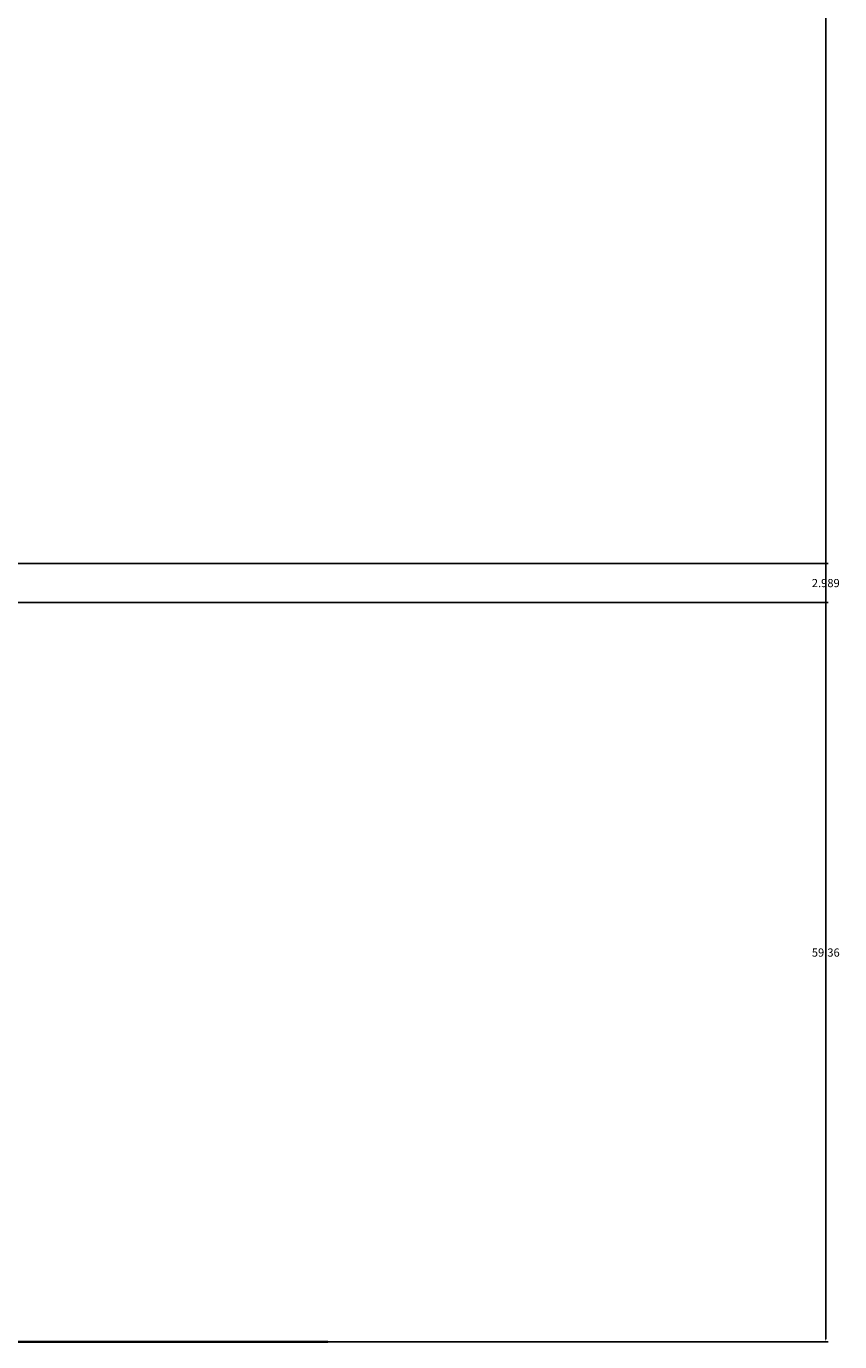
# Model space of a CAD drawing. Units: inches. Extents: x -13 to 809, y 112 to 656.
# Tile 45 of 55: x 747 to 809, y 151 to 251. Entities that reach past the tile are written whole.
import ezdxf

# ---------------------------------------------------------------- set-up
doc = ezdxf.new("R2010")
doc.units = ezdxf.units.IN
doc.header["$MEASUREMENT"] = 0
doc.layers.add('A-ANNO-DIMS', color=2, linetype='Continuous', lineweight=18)
doc.layers.add('A-ELEV', color=7, linetype='Continuous', lineweight=35)
doc.styles.get("Standard").update_dxf_attribs({"font": 'arial.ttf'})
doc.dimstyles.get("Standard").update_dxf_attribs({"dimtxt": 0.625, "dimasz": 0.18, "dimexe": 0.18, "dimexo": 0.0625, "dimgap": 0.09, "dimtad": 0, "dimtih": 1, "dimtoh": 1, "dimdec": 4, "dimzin": 0, "dimdsep": 46, "dimlunit": 4, "dimtxsty": 'Standard', "dimcen": 0.09, "dimadec": 0, "dimazin": 0, "dimtfac": 1, "dimtdec": 4, "dimtofl": 0, "dimtmove": 0, "dimatfit": 3, "dimfxl": 1, "dimtolj": 1, "dimtzin": 0, "dimarcsym": 0})

# ---------------------------------------------------------------- blocks, each defined once
blk = doc.blocks.new('*D31')
at = {"layer": 'A-ANNO-DIMS', "color": 0, "lineweight": -2, "transparency": 16777216}
for p, q in [((621.07, 617.78), (807.77, 617.78)), ((807.59, 617.6), (807.59, 384.56)), ((807.59, 150.7), (807.59, 383.74)), ((621.07, 150.52), (807.77, 150.52))]:
    blk.add_line(p, q, dxfattribs=at)
at = {"layer": 'A-ANNO-DIMS', "color": 0, "transparency": 16777216}
for points in [[(807.56, 617.6), (807.62, 617.6), (807.59, 617.78)], [(807.56, 150.7), (807.62, 150.7), (807.59, 150.52)]]:
    blk.add_solid(points, dxfattribs=at)
at = {"layer": 'Defpoints', "color": 0, "transparency": 16777216}
for p in [(621.01, 617.78), (807.59, 617.78), (621.01, 150.52)]:
    blk.add_point(p, dxfattribs=at)
at = {"layer": 'A-ANNO-DIMS', "color": 0, "transparency": 16777216, "insert": (807.59, 384.15), "char_height": 0.625, "attachment_point": 5}
blk.add_mtext('\\A1;467.3', dxfattribs=at)
blk = doc.blocks.new('*D129')
at = {"layer": 'A-ANNO-DIMS', "color": 0, "lineweight": -2, "transparency": 16777216}
for p, q in [((607.64, 209.88), (807.77, 209.88)), ((807.59, 209.7), (807.59, 180.61)), ((807.59, 150.7), (807.59, 179.79)), ((608.76, 150.52), (807.77, 150.52))]:
    blk.add_line(p, q, dxfattribs=at)
at = {"layer": 'A-ANNO-DIMS', "color": 0, "transparency": 16777216}
for points in [[(807.56, 209.7), (807.62, 209.7), (807.59, 209.88)], [(807.56, 150.7), (807.62, 150.7), (807.59, 150.52)]]:
    blk.add_solid(points, dxfattribs=at)
at = {"layer": 'Defpoints', "color": 0, "transparency": 16777216}
for p in [(607.57, 209.88), (807.59, 209.88), (608.69, 150.52)]:
    blk.add_point(p, dxfattribs=at)
at = {"layer": 'A-ANNO-DIMS', "color": 0, "transparency": 16777216, "insert": (807.59, 180.2), "char_height": 0.625, "attachment_point": 5}
blk.add_mtext('\\A1;59.36', dxfattribs=at)
blk = doc.blocks.new('*D132')
at = {"layer": 'A-ANNO-DIMS', "color": 0, "lineweight": -2, "transparency": 16777216}
for p, q in [((607.64, 209.88), (807.77, 209.88)), ((807.59, 209.7), (807.59, 208.79)), ((807.59, 207.07), (807.59, 207.97)), ((604.64, 206.89), (807.77, 206.89))]:
    blk.add_line(p, q, dxfattribs=at)
at = {"layer": 'A-ANNO-DIMS', "color": 0, "transparency": 16777216}
for points in [[(807.56, 209.7), (807.62, 209.7), (807.59, 209.88)], [(807.56, 207.07), (807.62, 207.07), (807.59, 206.89)]]:
    blk.add_solid(points, dxfattribs=at)
at = {"layer": 'Defpoints', "color": 0, "transparency": 16777216}
for p in [(607.57, 209.88), (807.59, 209.88), (604.57, 206.89)]:
    blk.add_point(p, dxfattribs=at)
at = {"layer": 'A-ANNO-DIMS', "color": 0, "transparency": 16777216, "insert": (807.59, 208.38), "char_height": 0.625, "attachment_point": 5}
blk.add_mtext('\\A1;2.989', dxfattribs=at)

msp = doc.modelspace()

# ---------------------------------------------------------------- linework, layer by layer
at = {"layer": 'A-ELEV'}
msp.add_line((649.5888, 150.5199), (769.5888, 150.5199), dxfattribs=at)

# ---------------------------------------------------------------- dimensions: what is measured, and where the dimension line sits
at = {"layer": 'A-ANNO-DIMS'}
for base, p1, p2, override, picture, middle in [((807.5888, 617.7828), (621.008, 150.5199), (621.008, 617.7828), {"dimdec": 1, "dimlfac": 1, "dimrnd": 0, "dimzin": 0, "dimdsep": 46, "dimlunit": 2}, '*D31', (807.5888, 384.1514)), ((807.5888, 209.8753), (604.5741, 206.8866), (607.5741, 209.8753), {"dimdec": 3, "dimlfac": 1, "dimrnd": 0, "dimzin": 0, "dimdsep": 46, "dimlunit": 2}, '*D132', (807.5888, 208.381)), ((807.5888, 209.8753), (608.694, 150.5199), (607.5741, 209.8753), {"dimdec": 2, "dimlfac": 1, "dimrnd": 0, "dimzin": 0, "dimdsep": 46, "dimlunit": 2}, '*D129', (807.5888, 180.1976))]:
    dim = msp.add_linear_dim(base=base, p1=p1, p2=p2, angle=90, dimstyle='Standard', override=override, dxfattribs=at)
    dim.commit()
    dim.dimension.update_dxf_attribs({"geometry": picture, "text_midpoint": middle})

doc.saveas('drawing.dxf')
